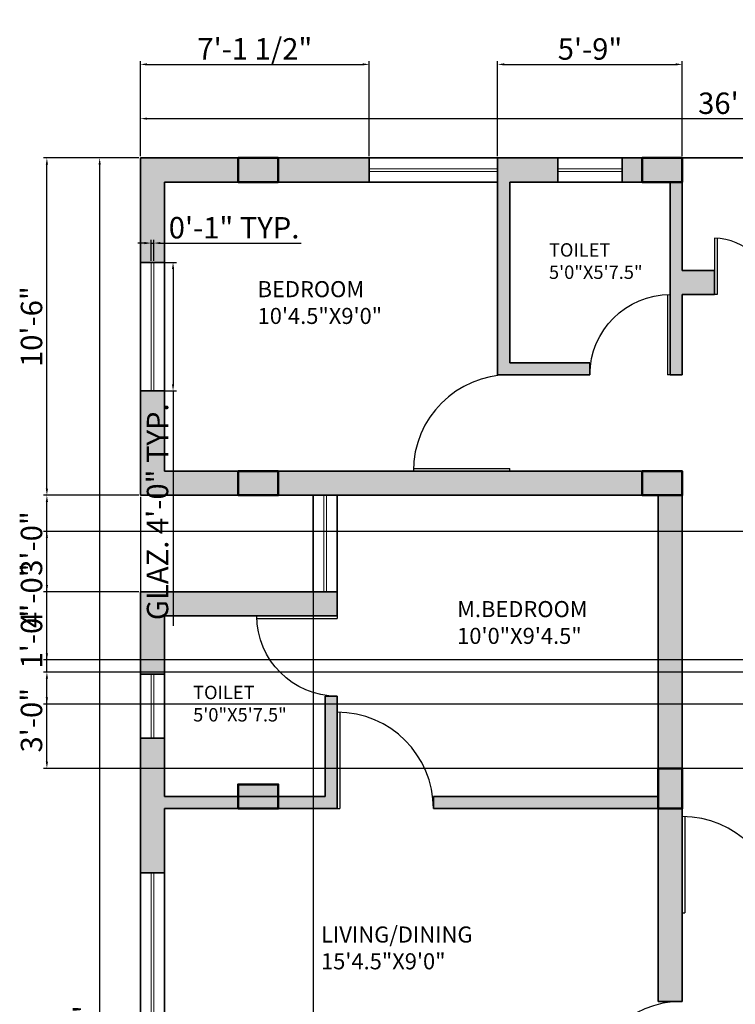
# Model space of a CAD drawing. Units: inches. Extents: x 3010 to 3575, y 2253 to 2995.
# Tile 3 of 4: x 3010 to 3278, y 2627 to 2995. Entities that reach past the tile are written whole.
import ezdxf

# ---------------------------------------------------------------- set-up
doc = ezdxf.new("R2010")
doc.units = ezdxf.units.IN
for name, color, linetype, lineweight in [('A-ANNO-DIMS', 2, 'Continuous', 18), ('A-AREA-IDEN', 7, 'Continuous', 18), ('A-COLS', 7, 'Continuous', 50), ('A-COLS-PATT', 1, 'Continuous', 13), ('A-DOOR', 3, 'Continuous', 25), ('A-GLAZ', 4, 'Continuous', 18), ('A-WALL', 7, 'Continuous', 35)]:
    doc.layers.add(name, color=color, linetype=linetype, lineweight=lineweight)
doc.layers.add('A-WALL-PATT', color=9, linetype='Continuous', lineweight=13, true_color=0xc7c8ca)
doc.styles.get("Standard").update_dxf_attribs({"font": 'arial.ttf'})
doc.dimstyles.new('ISO-25', dxfattribs={"dimtxt": 8, "dimasz": 2.5, "dimexe": 1.25, "dimexo": 0.625, "dimtad": 1, "dimdec": 1, "dimlunit": 3, "dimtxsty": 'Standard', "dimcen": 2.5, "dimadec": 0, "dimazin": 0, "dimtfac": 1, "dimtdec": 1, "dimtmove": 0, "dimatfit": 3, "dimfxl": 1, "dimarcsym": 0})

# ---------------------------------------------------------------- blocks, each defined once
blk = doc.blocks.new('*D1')
at = {"layer": 'A-ANNO-DIMS', "color": 0, "lineweight": -2, "transparency": 16777216}
for p, q in [((3055.45, 2944.01), (3055.45, 2959.31)), ((3057.95, 2958.06), (3484.95, 2958.06)), ((3487.45, 2944.01), (3487.45, 2959.31))]:
    blk.add_line(p, q, dxfattribs=at)
at = {"layer": 'A-ANNO-DIMS', "color": 0, "transparency": 16777216}
for points in [[(3057.95, 2958.48), (3057.95, 2957.65), (3055.45, 2958.06)], [(3484.95, 2958.48), (3484.95, 2957.65), (3487.45, 2958.06)]]:
    blk.add_solid(points, dxfattribs=at)
at = {"layer": 'Defpoints', "color": 0, "transparency": 16777216}
for p in [(3487.45, 2958.06), (3055.45, 2943.38), (3487.45, 2943.38)]:
    blk.add_point(p, dxfattribs=at)
at = {"layer": 'A-ANNO-DIMS', "color": 0, "transparency": 16777216, "insert": (3271.45, 2962.78), "char_height": 8, "attachment_point": 5}
blk.add_mtext("36'", dxfattribs=at)
blk = doc.blocks.new('*D2')
at = {"layer": 'A-ANNO-DIMS', "color": 0, "lineweight": -2, "transparency": 16777216}
for p, q in [((3054.82, 2943.38), (3038.98, 2943.38)), ((3040.23, 2297.88), (3040.23, 2940.88)), ((3054.82, 2295.38), (3038.98, 2295.38))]:
    blk.add_line(p, q, dxfattribs=at)
at = {"layer": 'A-ANNO-DIMS', "color": 0, "transparency": 16777216}
for points in [[(3039.81, 2940.88), (3040.64, 2940.88), (3040.23, 2943.38)], [(3039.81, 2297.88), (3040.64, 2297.88), (3040.23, 2295.38)]]:
    blk.add_solid(points, dxfattribs=at)
at = {"layer": 'Defpoints', "color": 0, "transparency": 16777216}
for p in [(3040.23, 2943.38), (3055.45, 2943.38), (3055.45, 2295.38)]:
    blk.add_point(p, dxfattribs=at)
at = {"layer": 'A-ANNO-DIMS', "color": 0, "transparency": 16777216, "insert": (3035.53, 2619.38), "char_height": 8, "attachment_point": 5, "rotation": 90}
blk.add_mtext("54'", dxfattribs=at)
blk = doc.blocks.new("D1 3'")
for p, q in [((0, 36), (0, 0)), ((1, 36), (1, 0)), ((0, 0), (1, 0))]:
    blk.add_line(p, q)
blk.add_arc((0, 0), 36, 0, 90)
blk = doc.blocks.new("D2 2'6")
for p, q in [((0, 30), (0, 0)), ((1, 30), (1, 0)), ((0, 0), (1, 0))]:
    blk.add_line(p, q)
blk.add_arc((0, 0), 30, 0, 90)
blk = doc.blocks.new('FLOD D')
for p, q in [((3539.49, 2401.61), (3539.49, 2380.61)), ((3540.49, 2401.61), (3540.49, 2380.61)), ((3560.49, 2401.61), (3560.49, 2380.61)), ((3561.49, 2401.61), (3561.49, 2380.61)), ((3601.49, 2401.61), (3601.49, 2380.61)), ((3602.49, 2401.61), (3602.49, 2380.61)), ((3622.49, 2401.61), (3622.49, 2380.61)), ((3623.49, 2401.61), (3623.49, 2380.61)), ((3540.49, 2380.61), (3539.49, 2380.61)), ((3561.49, 2380.61), (3560.49, 2380.61)), ((3602.49, 2380.61), (3601.49, 2380.61)), ((3623.49, 2380.61), (3622.49, 2380.61))]:
    blk.add_line(p, q)
for centre, start, end in [((3539.49, 2380.61), 0, 90), ((3560.49, 2380.61), 0, 90), ((3602.49, 2380.61), 90, 180), ((3623.49, 2380.61), 90, 180)]:
    blk.add_arc(centre, 21, start, end)
blk = doc.blocks.new('GLAZING-24IN')
for p, q in [((24, 1), (0, 1)), ((24, 0), (0, 0))]:
    blk.add_line(p, q)
blk = doc.blocks.new('GLAZING-36IN')
for p, q in [((36, 1), (0, 1)), ((36, 0), (0, 0))]:
    blk.add_line(p, q)
blk = doc.blocks.new('GLAZING-48IN')
for p, q in [((48, 1), (0, 1)), ((48, 0), (0, 0))]:
    blk.add_line(p, q)
blk = doc.blocks.new('GLAZING-60IN')
for p, q in [((0, 0), (0, 60)), ((1, 0), (1, 60))]:
    blk.add_line(p, q)
blk = doc.blocks.new('*D19')
at = {"layer": 'A-ANNO-DIMS', "color": 0, "lineweight": -2, "transparency": 16777216}
for p, q in [((3061.07, 2904.38), (3068.9, 2904.38)), ((3067.65, 2901.88), (3067.65, 2858.88)), ((3061.07, 2856.38), (3068.9, 2856.38)), ((3067.65, 2856.38), (3067.65, 2768.6))]:
    blk.add_line(p, q, dxfattribs=at)
at = {"layer": 'A-ANNO-DIMS', "color": 0, "transparency": 16777216}
for points in [[(3067.23, 2901.88), (3068.06, 2901.88), (3067.65, 2904.38)], [(3067.23, 2858.88), (3068.06, 2858.88), (3067.65, 2856.38)]]:
    blk.add_solid(points, dxfattribs=at)
at = {"layer": 'Defpoints', "color": 0, "transparency": 16777216}
for p in [(3060.45, 2904.38), (3060.45, 2856.38), (3067.65, 2856.38)]:
    blk.add_point(p, dxfattribs=at)
at = {"layer": 'A-ANNO-DIMS', "color": 0, "transparency": 16777216, "insert": (3062.88, 2811.24), "char_height": 8, "attachment_point": 5, "rotation": 90}
blk.add_mtext('GLAZ. 4\'-0" TYP.', dxfattribs=at)
blk = doc.blocks.new('*D20')
at = {"layer": 'A-ANNO-DIMS', "color": 0, "lineweight": -2, "transparency": 16777216}
for p, q in [((3059.45, 2905.01), (3059.45, 2912.83)), ((3060.45, 2905.01), (3060.45, 2912.83)), ((3056.95, 2911.58), (3054.45, 2911.58)), ((3059.45, 2911.58), (3060.45, 2911.58)), ((3062.95, 2911.58), (3115.46, 2911.58))]:
    blk.add_line(p, q, dxfattribs=at)
at = {"layer": 'A-ANNO-DIMS', "color": 0, "transparency": 16777216}
for points in [[(3056.95, 2912), (3056.95, 2911.17), (3059.45, 2911.58)], [(3062.95, 2912), (3062.95, 2911.17), (3060.45, 2911.58)]]:
    blk.add_solid(points, dxfattribs=at)
at = {"layer": 'Defpoints', "color": 0, "transparency": 16777216}
for p in [(3060.45, 2911.58), (3059.45, 2904.38), (3060.45, 2904.38)]:
    blk.add_point(p, dxfattribs=at)
at = {"layer": 'A-ANNO-DIMS', "color": 0, "transparency": 16777216, "insert": (3090.45, 2916.29), "char_height": 8, "attachment_point": 5}
blk.add_mtext('0\'-1" TYP.', dxfattribs=at)
blk = doc.blocks.new('*D40')
at = {"layer": 'A-ANNO-DIMS', "color": 0, "lineweight": -2, "transparency": 16777216}
for p, q in [((3389.32, 2803.88), (3019.25, 2803.88)), ((3020.5, 2758.38), (3020.5, 2801.38)), ((3389.32, 2755.88), (3019.25, 2755.88))]:
    blk.add_line(p, q, dxfattribs=at)
at = {"layer": 'A-ANNO-DIMS', "color": 0, "transparency": 16777216}
for points in [[(3020.08, 2801.38), (3020.91, 2801.38), (3020.5, 2803.88)], [(3020.08, 2758.38), (3020.91, 2758.38), (3020.5, 2755.88)]]:
    blk.add_solid(points, dxfattribs=at)
at = {"layer": 'Defpoints', "color": 0, "transparency": 16777216}
for p in [(3020.5, 2803.88), (3389.95, 2803.88), (3389.95, 2755.88)]:
    blk.add_point(p, dxfattribs=at)
at = {"layer": 'A-ANNO-DIMS', "color": 0, "transparency": 16777216, "insert": (3015.79, 2779.88), "char_height": 8, "attachment_point": 5, "rotation": 90}
blk.add_mtext('4\'-0"', dxfattribs=at)
blk = doc.blocks.new('*D42')
at = {"layer": 'A-ANNO-DIMS', "color": 0, "lineweight": -2, "transparency": 16777216}
for p, q in [((3365.32, 2751.38), (3019.25, 2751.38)), ((3020.5, 2717.88), (3020.5, 2748.88)), ((3365.32, 2715.38), (3019.25, 2715.38))]:
    blk.add_line(p, q, dxfattribs=at)
at = {"layer": 'A-ANNO-DIMS', "color": 0, "transparency": 16777216}
for points in [[(3020.08, 2748.88), (3020.91, 2748.88), (3020.5, 2751.38)], [(3020.08, 2717.88), (3020.91, 2717.88), (3020.5, 2715.38)]]:
    blk.add_solid(points, dxfattribs=at)
at = {"layer": 'Defpoints', "color": 0, "transparency": 16777216}
for p in [(3020.5, 2751.38), (3365.95, 2751.38), (3365.95, 2715.38)]:
    blk.add_point(p, dxfattribs=at)
at = {"layer": 'A-ANNO-DIMS', "color": 0, "transparency": 16777216, "insert": (3015.78, 2733.38), "char_height": 8, "attachment_point": 5, "rotation": 90}
blk.add_mtext('3\'-0"', dxfattribs=at)
blk = doc.blocks.new('*D43')
at = {"layer": 'A-ANNO-DIMS', "color": 0, "lineweight": -2, "transparency": 16777216}
for p, q in [((3020.5, 2751.38), (3020.5, 2775.65)), ((3411.82, 2751.38), (3019.25, 2751.38)), ((3020.5, 2741.88), (3020.5, 2748.88)), ((3416.32, 2739.38), (3019.25, 2739.38))]:
    blk.add_line(p, q, dxfattribs=at)
at = {"layer": 'A-ANNO-DIMS', "color": 0, "transparency": 16777216}
for points in [[(3020.08, 2748.88), (3020.91, 2748.88), (3020.5, 2751.38)], [(3020.08, 2741.88), (3020.91, 2741.88), (3020.5, 2739.38)]]:
    blk.add_solid(points, dxfattribs=at)
at = {"layer": 'Defpoints', "color": 0, "transparency": 16777216}
for p in [(3020.5, 2751.38), (3412.45, 2751.38), (3416.95, 2739.38)]:
    blk.add_point(p, dxfattribs=at)
at = {"layer": 'A-ANNO-DIMS', "color": 0, "transparency": 16777216, "insert": (3015.79, 2764.76), "char_height": 8, "attachment_point": 5, "rotation": 90}
blk.add_mtext('1\'-0"', dxfattribs=at)
blk = doc.blocks.new('*D48')
at = {"layer": 'A-ANNO-DIMS', "color": 0, "lineweight": -2, "transparency": 16777216}
for p, q in [((3188.95, 2944.01), (3188.95, 2979.58)), ((3257.95, 2944.01), (3257.95, 2979.58)), ((3191.45, 2978.33), (3255.45, 2978.33))]:
    blk.add_line(p, q, dxfattribs=at)
at = {"layer": 'A-ANNO-DIMS', "color": 0, "transparency": 16777216}
for points in [[(3191.45, 2978.75), (3191.45, 2977.92), (3188.95, 2978.33)], [(3255.45, 2978.75), (3255.45, 2977.92), (3257.95, 2978.33)]]:
    blk.add_solid(points, dxfattribs=at)
at = {"layer": 'Defpoints', "color": 0, "transparency": 16777216}
for p in [(3257.95, 2978.33), (3188.95, 2943.38), (3257.95, 2943.38)]:
    blk.add_point(p, dxfattribs=at)
at = {"layer": 'A-ANNO-DIMS', "color": 0, "transparency": 16777216, "insert": (3223.45, 2983.04), "char_height": 8, "attachment_point": 5}
blk.add_mtext('5\'-9"', dxfattribs=at)
blk = doc.blocks.new('*D51')
at = {"layer": 'A-ANNO-DIMS', "color": 0, "lineweight": -2, "transparency": 16777216}
for p, q in [((3054.82, 2943.38), (3019.25, 2943.38)), ((3020.5, 2819.88), (3020.5, 2940.88)), ((3054.82, 2817.38), (3019.25, 2817.38))]:
    blk.add_line(p, q, dxfattribs=at)
at = {"layer": 'A-ANNO-DIMS', "color": 0, "transparency": 16777216}
for points in [[(3020.08, 2940.88), (3020.91, 2940.88), (3020.5, 2943.38)], [(3020.08, 2819.88), (3020.91, 2819.88), (3020.5, 2817.38)]]:
    blk.add_solid(points, dxfattribs=at)
at = {"layer": 'Defpoints', "color": 0, "transparency": 16777216}
for p in [(3020.5, 2943.38), (3055.45, 2943.38), (3055.45, 2817.38)]:
    blk.add_point(p, dxfattribs=at)
at = {"layer": 'A-ANNO-DIMS', "color": 0, "transparency": 16777216, "insert": (3015.79, 2880.38), "char_height": 8, "attachment_point": 5, "rotation": 90}
blk.add_mtext('10\'-6"', dxfattribs=at)
blk = doc.blocks.new('*D52')
at = {"layer": 'A-ANNO-DIMS', "color": 0, "lineweight": -2, "transparency": 16777216}
for p, q in [((3054.82, 2817.38), (3019.25, 2817.38)), ((3020.5, 2783.88), (3020.5, 2814.88)), ((3054.82, 2781.38), (3019.25, 2781.38))]:
    blk.add_line(p, q, dxfattribs=at)
at = {"layer": 'A-ANNO-DIMS', "color": 0, "transparency": 16777216}
for points in [[(3020.08, 2814.88), (3020.91, 2814.88), (3020.5, 2817.38)], [(3020.08, 2783.88), (3020.91, 2783.88), (3020.5, 2781.38)]]:
    blk.add_solid(points, dxfattribs=at)
at = {"layer": 'Defpoints', "color": 0, "transparency": 16777216}
for p in [(3020.5, 2817.38), (3055.45, 2817.38), (3055.45, 2781.38)]:
    blk.add_point(p, dxfattribs=at)
at = {"layer": 'A-ANNO-DIMS', "color": 0, "transparency": 16777216, "insert": (3015.78, 2799.38), "char_height": 8, "attachment_point": 5, "rotation": 90}
blk.add_mtext('3\'-0"', dxfattribs=at)
blk = doc.blocks.new('*D53')
at = {"layer": 'A-ANNO-DIMS', "color": 0, "lineweight": -2, "transparency": 16777216}
for p, q in [((3055.45, 2816.76), (3055.45, 2259.18)), ((3119.95, 2816.76), (3119.95, 2259.18)), ((3057.95, 2260.43), (3117.45, 2260.43))]:
    blk.add_line(p, q, dxfattribs=at)
at = {"layer": 'A-ANNO-DIMS', "color": 0, "transparency": 16777216}
for points in [[(3057.95, 2260.85), (3057.95, 2260.02), (3055.45, 2260.43)], [(3117.45, 2260.85), (3117.45, 2260.02), (3119.95, 2260.43)]]:
    blk.add_solid(points, dxfattribs=at)
at = {"layer": 'Defpoints', "color": 0, "transparency": 16777216}
for p in [(3055.45, 2817.38), (3119.95, 2817.38), (3119.95, 2260.43)]:
    blk.add_point(p, dxfattribs=at)
at = {"layer": 'A-ANNO-DIMS', "color": 0, "transparency": 16777216, "insert": (3087.7, 2265.19), "char_height": 8, "attachment_point": 5}
blk.add_mtext('5\'-4 1/2"', dxfattribs=at)
blk = doc.blocks.new('*D55')
at = {"layer": 'A-ANNO-DIMS', "color": 0, "lineweight": -2, "transparency": 16777216}
for p, q in [((3055.45, 2944.01), (3055.45, 2979.58)), ((3140.95, 2944.01), (3140.95, 2979.58)), ((3057.95, 2978.33), (3138.45, 2978.33))]:
    blk.add_line(p, q, dxfattribs=at)
at = {"layer": 'A-ANNO-DIMS', "color": 0, "transparency": 16777216}
for points in [[(3057.95, 2978.75), (3057.95, 2977.92), (3055.45, 2978.33)], [(3138.45, 2978.75), (3138.45, 2977.92), (3140.95, 2978.33)]]:
    blk.add_solid(points, dxfattribs=at)
at = {"layer": 'Defpoints', "color": 0, "transparency": 16777216}
for p in [(3140.95, 2978.33), (3055.45, 2943.38), (3140.95, 2943.38)]:
    blk.add_point(p, dxfattribs=at)
at = {"layer": 'A-ANNO-DIMS', "color": 0, "transparency": 16777216, "insert": (3098.2, 2983.09), "char_height": 8, "attachment_point": 5}
blk.add_mtext('7\'-1 1/2"', dxfattribs=at)

msp = doc.modelspace()

# ---------------------------------------------------------------- hatches: boundary and pattern name
at = {"layer": 'A-COLS-PATT'}
h = msp.add_hatch(color=256, dxfattribs=at)
h.dxf.hatch_style = 1
h.paths.add_polyline_path([(3106.95, 2934.38), (3106.95, 2943.38), (3091.95, 2943.38), (3091.95, 2934.38)])
h = msp.add_hatch(color=256, dxfattribs=at)
h.dxf.hatch_style = 1
h.paths.add_polyline_path([(3257.95, 2934.38), (3257.95, 2943.38), (3242.95, 2943.38), (3242.95, 2934.38)])
h = msp.add_hatch(color=256, dxfattribs=at)
h.dxf.hatch_style = 1
h.paths.add_polyline_path([(3106.95, 2817.38), (3106.95, 2826.38), (3091.95, 2826.38), (3091.95, 2817.38)])
h = msp.add_hatch(color=256, dxfattribs=at)
h.dxf.hatch_style = 1
h.paths.add_polyline_path([(3257.95, 2817.38), (3257.95, 2826.38), (3242.95, 2826.38), (3242.95, 2817.38)])
h = msp.add_hatch(color=256, dxfattribs=at)
h.dxf.hatch_style = 1
h.paths.add_polyline_path([(3248.95, 2700.38), (3257.95, 2700.38), (3257.95, 2715.38), (3248.95, 2715.38)])
h = msp.add_hatch(color=256, dxfattribs=at)
h.dxf.hatch_style = 1
h.paths.add_polyline_path([(3106.95, 2700.38), (3106.95, 2709.38), (3091.95, 2709.38), (3091.95, 2700.38)])
at = {"layer": 'A-WALL-PATT', "transparency": 33554687}
h = msp.add_hatch(color=256, dxfattribs=at)
h.dxf.hatch_style = 1
h.paths.add_polyline_path([(3064.45, 2499.38), (3055.45, 2499.38), (3055.45, 2457.38), (3064.45, 2457.38)])
h.paths.add_polyline_path([(3091.95, 2421.38), (3055.45, 2421.38), (3055.45, 2382.38), (3064.45, 2382.38), (3064.45, 2412.38), (3091.95, 2412.38)])
h.paths.add_polyline_path([(3248.95, 2421.38), (3176.95, 2421.38), (3176.95, 2464.88), (3194.99, 2464.88), (3194.99, 2473.88), (3176.95, 2473.88), (3176.95, 2551.88), (3172.45, 2551.88), (3172.45, 2515.88), (3172.45, 2421.38), (3106.95, 2421.38), (3106.95, 2412.38), (3248.95, 2412.38)])
h.paths.add_polyline_path([(3064.45, 2346.38), (3055.45, 2346.38), (3055.45, 2295.38), (3091.95, 2295.38), (3091.95, 2304.38), (3064.45, 2304.38)])
h.paths.add_polyline_path([(3129.95, 2304.38), (3106.95, 2304.38), (3106.95, 2295.38), (3129.95, 2295.38)])
h.paths.add_polyline_path([(3211.45, 2304.38), (3193.45, 2304.38), (3193.45, 2376.88), (3188.95, 2376.88), (3188.95, 2304.38), (3165.95, 2304.38), (3165.95, 2295.38), (3211.45, 2295.38)])
h.paths.add_polyline_path([(3269.95, 2346.38), (3257.95, 2346.38), (3257.95, 2376.88), (3223.45, 2376.88), (3223.45, 2371.88), (3253.45, 2371.88), (3253.45, 2304.38), (3257.95, 2304.38), (3257.95, 2337.38), (3269.95, 2337.38)])
h.paths.add_polyline_path([(3242.95, 2304.38), (3235.45, 2304.38), (3235.45, 2295.38), (3242.95, 2295.38)])
h.paths.add_polyline_path([(3370.45, 2346.38), (3353.95, 2346.38), (3353.95, 2337.38), (3365.95, 2337.38), (3365.95, 2304.38), (3370.45, 2304.38)])
h.paths.add_polyline_path([(3389.94, 2304.38), (3380.95, 2304.38), (3380.95, 2295.38), (3389.94, 2295.38)], flags=17)
h.paths.add_polyline_path([(3435.95, 2304.38), (3425.94, 2304.38), (3425.94, 2295.38), (3435.95, 2295.38)], flags=17)
h.paths.add_polyline_path([(3487.45, 2401.88), (3478.45, 2401.88), (3478.45, 2389.88), (3394.45, 2389.88), (3394.45, 2442.38), (3380.95, 2442.38), (3380.95, 2437.88), (3389.95, 2437.88), (3389.95, 2389.88), (3365.95, 2389.88), (3365.95, 2385.38), (3412.45, 2385.38), (3412.45, 2373.38), (3416.95, 2373.38), (3416.95, 2385.38), (3478.45, 2385.38), (3478.45, 2304.38), (3450.95, 2304.38), (3450.95, 2295.38), (3487.45, 2295.38)])
h.paths.add_polyline_path([(3487.45, 2478.38), (3478.45, 2478.38), (3478.45, 2442.38), (3450.95, 2442.38), (3450.95, 2437.88), (3478.45, 2437.88), (3478.45, 2425.88), (3487.45, 2425.88)])
h.paths.add_polyline_path([(3435.95, 2442.38), (3424.45, 2442.38), (3424.45, 2437.88), (3435.95, 2437.88)], flags=17)
h.paths.add_polyline_path([(3248.95, 2592.38), (3221.95, 2592.38), (3172.45, 2592.38), (3172.45, 2587.88), (3248.95, 2587.88)])
h.paths.add_polyline_path([(3257.95, 2577.38), (3248.95, 2577.38), (3248.95, 2473.88), (3230.99, 2473.88), (3230.99, 2464.88), (3248.95, 2464.88), (3248.95, 2427.38), (3257.95, 2427.38)])
h.paths.add_polyline_path([(3365.95, 2583.38), (3293.95, 2583.38), (3293.95, 2574.38), (3365.95, 2574.38)])
h.paths.add_polyline_path([(3370.45, 2574.38), (3365.95, 2574.38), (3365.95, 2478.38), (3370.45, 2478.38)])
h.paths.add_polyline_path([(3435.95, 2583.38), (3380.95, 2583.38), (3380.95, 2574.38), (3435.95, 2574.38)])
h.paths.add_polyline_path([(3487.45, 2583.38), (3450.95, 2583.38), (3450.95, 2574.38), (3478.45, 2574.38), (3478.45, 2538.38), (3487.45, 2538.38)])
h.paths.add_polyline_path([(3064.45, 2551.88), (3055.45, 2551.88), (3055.45, 2535.38), (3136.45, 2535.38), (3136.45, 2557.88), (3131.95, 2557.88), (3131.95, 2539.88), (3064.45, 2539.88)])
h.paths.add_polyline_path([(3091.95, 2704.88), (3064.45, 2704.88), (3064.45, 2726.63), (3055.45, 2726.63), (3055.45, 2676.38), (3064.45, 2676.38), (3064.45, 2700.38), (3091.95, 2700.38)])
h.paths.add_polyline_path([(3064.45, 2616.38), (3055.45, 2616.38), (3055.45, 2575.88), (3064.45, 2575.88), (3064.45, 2587.88), (3091.95, 2587.88), (3091.95, 2592.38), (3064.45, 2592.38)])
h.paths.add_polyline_path([(3487.45, 2688.38), (3478.45, 2688.38), (3478.45, 2670.38), (3450.95, 2670.38), (3450.95, 2661.38), (3487.45, 2661.38)])
h.paths.add_polyline_path([(3450.95, 2661.38), (3446.45, 2661.38), (3446.45, 2583.38), (3450.95, 2583.38)])
h.paths.add_polyline_path([(3435.95, 2670.38), (3380.95, 2670.38), (3380.95, 2661.38), (3435.95, 2661.38)])
h.paths.add_polyline_path([(3365.95, 2670.38), (3293.95, 2670.38), (3293.95, 2661.38), (3365.95, 2661.38)])
h.paths.add_polyline_path([(3370.45, 2715.38), (3365.95, 2715.38), (3365.95, 2670.38), (3370.45, 2670.38)])
h.paths.add_polyline_path([(3257.95, 2700.38), (3248.95, 2700.38), (3248.95, 2628.38), (3257.95, 2628.38)])
h.paths.add_polyline_path([(3128.95, 2742.38), (3124.45, 2742.38), (3124.45, 2704.88), (3106.95, 2704.88), (3106.95, 2700.38), (3128.95, 2700.38)])
h.paths.add_polyline_path([(3248.95, 2704.88), (3164.95, 2704.88), (3164.95, 2700.38), (3248.95, 2700.38)])
h.paths.add_polyline_path([(3257.95, 2817.38), (3248.95, 2817.38), (3248.95, 2715.38), (3257.95, 2715.38)])
h.paths.add_polyline_path([(3128.95, 2781.38), (3055.45, 2781.38), (3055.45, 2750.63), (3064.45, 2750.63), (3064.45, 2772.38), (3128.95, 2772.38)])
h.paths.add_polyline_path([(3242.95, 2826.38), (3106.95, 2826.38), (3106.95, 2817.38), (3242.95, 2817.38)])
h.paths.add_polyline_path([(3091.95, 2826.38), (3064.45, 2826.38), (3064.45, 2856.38), (3055.45, 2856.38), (3055.45, 2817.38), (3091.95, 2817.38)])
h.paths.add_polyline_path([(3064.45, 2934.38), (3091.95, 2934.38), (3091.95, 2943.38), (3055.45, 2943.38), (3055.45, 2904.38), (3064.45, 2904.38)])
h.paths.add_polyline_path([(3140.95, 2943.38), (3106.95, 2943.38), (3106.95, 2934.38), (3140.95, 2934.38)])
h.paths.add_polyline_path([(3211.45, 2943.38), (3188.95, 2943.38), (3188.95, 2862.38), (3223.45, 2862.38), (3223.45, 2866.88), (3193.45, 2866.88), (3193.45, 2934.38), (3211.45, 2934.38)])
h.paths.add_polyline_path([(3257.95, 2934.38), (3253.45, 2934.38), (3253.45, 2862.38), (3257.95, 2862.38), (3257.95, 2892.38), (3269.95, 2892.38), (3269.95, 2901.38), (3257.95, 2901.38)])
h.paths.add_polyline_path([(3242.95, 2943.38), (3235.45, 2943.38), (3235.45, 2934.38), (3242.95, 2934.38)])
h.paths.add_polyline_path([(3370.45, 2934.38), (3365.95, 2934.38), (3365.95, 2901.38), (3353.95, 2901.38), (3353.95, 2892.38), (3365.95, 2892.38), (3365.95, 2844.38), (3370.45, 2844.38)])
h.paths.add_polyline_path([(3389.94, 2943.38), (3380.95, 2943.38), (3380.95, 2934.38), (3389.94, 2934.38)])
h.paths.add_polyline_path([(3435.95, 2943.38), (3425.94, 2943.38), (3425.94, 2934.38), (3435.95, 2934.38)])
h.paths.add_polyline_path([(3487.45, 2943.38), (3450.95, 2943.38), (3450.95, 2934.38), (3478.45, 2934.38), (3478.45, 2895.38), (3487.45, 2895.38)])
h.paths.add_polyline_path([(3487.45, 2847.38), (3478.45, 2847.38), (3478.45, 2808.38), (3450.95, 2808.38), (3450.95, 2803.88), (3478.45, 2803.88), (3478.45, 2791.88), (3487.45, 2791.88)])
h.paths.add_polyline_path([(3435.95, 2808.38), (3424.45, 2808.38), (3424.45, 2803.88), (3435.95, 2803.88)])
h.paths.add_polyline_path([(3487.45, 2767.88), (3478.45, 2767.88), (3478.45, 2755.88), (3394.45, 2755.88), (3394.45, 2808.38), (3380.95, 2808.38), (3380.95, 2803.88), (3389.95, 2803.88), (3389.95, 2755.88), (3365.95, 2755.88), (3365.95, 2751.38), (3412.45, 2751.38), (3412.45, 2739.38), (3416.95, 2739.38), (3416.95, 2751.38), (3478.45, 2751.38), (3478.45, 2724.38), (3487.45, 2724.38)])
h.paths.add_polyline_path([(3398.97, 2495.84), (3456.57, 2495.84), (3456.57, 2518.66), (3398.97, 2518.66)], flags=9)

# ---------------------------------------------------------------- linework, layer by layer
at = {"layer": 'A-COLS'}
for points in [[(3091.95, 2934.38), (3091.95, 2943.38), (3106.95, 2943.38), (3106.95, 2934.38)], [(3242.95, 2934.38), (3242.95, 2943.38), (3257.95, 2943.38), (3257.95, 2934.38)], [(3091.95, 2817.38), (3091.95, 2826.38), (3106.95, 2826.38), (3106.95, 2817.38)], [(3242.95, 2817.38), (3242.95, 2826.38), (3257.95, 2826.38), (3257.95, 2817.38)], [(3248.95, 2715.38), (3257.95, 2715.38), (3257.95, 2700.38), (3248.95, 2700.38)], [(3091.95, 2700.38), (3091.95, 2709.38), (3106.95, 2709.38), (3106.95, 2700.38)]]:
    msp.add_lwpolyline(points, close=True, dxfattribs=at)
at = {"layer": 'A-WALL'}
for p, q in [((3055.45, 2943.38), (3487.45, 2943.38)), ((3055.45, 2817.38), (3055.45, 2943.38)), ((3140.95, 2934.38), (3140.95, 2943.38)), ((3188.95, 2862.38), (3188.95, 2943.38)), ((3211.45, 2934.38), (3211.45, 2943.38)), ((3235.45, 2934.38), (3235.45, 2943.38)), ((3257.95, 2901.38), (3257.95, 2943.38)), ((3064.45, 2934.38), (3188.95, 2934.38)), ((3064.45, 2826.38), (3064.45, 2934.38)), ((3193.45, 2934.38), (3253.45, 2934.38)), ((3193.45, 2866.88), (3193.45, 2934.38)), ((3253.45, 2862.38), (3253.45, 2934.38)), ((3064.45, 2904.38), (3055.45, 2904.38)), ((3257.95, 2901.38), (3269.95, 2901.38)), ((3269.95, 2892.38), (3269.95, 2901.38)), ((3257.95, 2862.38), (3257.95, 2892.38)), ((3257.95, 2892.38), (3269.95, 2892.38)), ((3193.45, 2866.88), (3223.45, 2866.88)), ((3223.45, 2862.38), (3223.45, 2866.88)), ((3188.95, 2862.38), (3223.45, 2862.38)), ((3253.45, 2862.38), (3257.95, 2862.38)), ((3064.45, 2856.38), (3055.45, 2856.38)), ((3064.45, 2826.38), (3257.95, 2826.38)), ((3257.95, 2628.38), (3257.95, 2826.38)), ((3055.45, 2817.38), (3248.95, 2817.38)), ((3119.95, 2781.38), (3119.95, 2817.38)), ((3128.95, 2772.38), (3128.95, 2817.38)), ((3248.95, 2704.88), (3248.95, 2817.38)), ((3055.45, 2781.38), (3128.95, 2781.38)), ((3055.45, 2535.38), (3055.45, 2781.38)), ((3064.45, 2704.88), (3064.45, 2772.38)), ((3064.45, 2772.38), (3128.95, 2772.38)), ((3064.45, 2750.63), (3055.45, 2750.63)), ((3124.45, 2704.88), (3124.45, 2742.38)), ((3124.45, 2742.38), (3128.95, 2742.38)), ((3128.95, 2700.38), (3128.95, 2742.38)), ((3064.45, 2726.63), (3055.45, 2726.63)), ((3064.45, 2704.88), (3124.45, 2704.88)), ((3164.95, 2700.38), (3164.95, 2704.88)), ((3164.95, 2704.88), (3248.95, 2704.88)), ((3064.45, 2700.38), (3128.95, 2700.38)), ((3064.45, 2592.38), (3064.45, 2700.38)), ((3164.95, 2700.38), (3248.95, 2700.38)), ((3248.95, 2628.38), (3248.95, 2700.38)), ((3064.45, 2676.38), (3055.45, 2676.38)), ((3248.95, 2628.38), (3257.95, 2628.38))]:
    msp.add_line(p, q, dxfattribs=at)

# ---------------------------------------------------------------- block references
at = {"layer": 'A-DOOR'}
for name, p in [('FLOD D', (-269.55, 511.77)), ("D1 3'", (3128.95, 2700.38)), ("D1 3'", (3257.95, 2661.38))]:
    msp.add_blockref(name, p, dxfattribs=at)
at = {"layer": 'A-DOOR', "xscale": -1}
msp.add_blockref("D2 2'6", (3253.45, 2862.38), dxfattribs=at)
at = {"layer": 'A-DOOR', "rotation": 90}
for p in [(3193.45, 2826.38), (3257.95, 2592.38)]:
    msp.add_blockref("D1 3'", p, dxfattribs=at)
at = {"layer": 'A-DOOR', "xscale": -1, "rotation": 90}
msp.add_blockref("D2 2'6", (3128.95, 2772.38), dxfattribs=at)
at = {"layer": 'A-GLAZ'}
for name, p in [('GLAZING-48IN', (3140.95, 2938.38)), ('GLAZING-24IN', (3211.45, 2938.38)), ('GLAZING-60IN', (3059.45, 2616.38))]:
    msp.add_blockref(name, p, dxfattribs=at)
for name, p, rotation in [('GLAZING-48IN', (3059.45, 2904.38), 269.9999999999989), ('GLAZING-36IN', (3123.95, 2817.38), 269.9999999999986), ('GLAZING-24IN', (3059.45, 2750.63), 270.0000000000001)]:
    msp.add_blockref(name, p, dxfattribs=dict(at, rotation=rotation))

# ---------------------------------------------------------------- texts
at = {"layer": 'A-AREA-IDEN', "attachment_point": 1}
for s, insert, char_height in [('{\\fTimes New Roman|b0|i0|c0|p18;\\P  TOILET\\P  5\'0"X5\'7.5"}', (3205.06, 2919.87), 5), ('{\\fTimes New Roman|b0|i0|c0|p18;\\PBEDROOM \\P10\'4.5"X9\'0"}', (3099.24, 2907.39), 6), ('{\\fTimes New Roman|b0|i0|c0|p18;\\PM.BEDROOM \\P10\'0"X9\'4.5"}', (3173.81, 2787.89), 6), ('{\\fTimes New Roman|b0|i0|c0|p18;\\P  TOILET\\P  5\'0"X5\'7.5"}', (3072.09, 2754.58), 5), ('{\\fTimes New Roman|b0|i0|c0|p18;\\PLIVING/DINING\\P15\'4.5"X9\'0"}', (3122.94, 2666.34), 6)]:
    msp.add_mtext_dynamic_manual_height_columns(s, width=72.5587, gutter_width=12.5, heights=[0], dxfattribs=dict(at, insert=insert, char_height=char_height))

# ---------------------------------------------------------------- dimensions: what is measured, and where the dimension line sits
at = {"layer": 'A-ANNO-DIMS'}
for base, p1, p2, override, picture, middle in [((3140.95, 2978.33), (3055.45, 2943.38), (3140.95, 2943.38), {"dimdec": 1, "dimlfac": 1, "dimrnd": 0, "dimzin": 1, "dimdsep": 46, "dimlunit": 4, "dimfrac": 2}, '*D55', (3098.2, 2983.09)), ((3257.95, 2978.33), (3188.95, 2943.38), (3257.95, 2943.38), {"dimdec": 1, "dimlfac": 1, "dimrnd": 0, "dimzin": 1, "dimdsep": 46, "dimlunit": 4, "dimfrac": 2}, '*D48', (3223.45, 2983.04)), ((3487.45, 2958.06), (3055.45, 2943.38), (3487.45, 2943.38), {"dimclrd": 0, "dimclre": 0, "dimclrt": 0}, '*D1', (3271.45, 2962.78)), ((3119.95, 2260.43), (3055.45, 2817.38), (3119.95, 2817.38), {"dimdec": 1, "dimlfac": 1, "dimrnd": 0, "dimzin": 1, "dimdsep": 46, "dimlunit": 4, "dimfrac": 2}, '*D53', (3087.7, 2265.19))]:
    dim = msp.add_linear_dim(base=base, p1=p1, p2=p2, dimstyle='ISO-25', override=override, dxfattribs=at)
    dim.commit()
    dim.dimension.update_dxf_attribs({"geometry": picture, "text_midpoint": middle})
for base, p1, p2, angle, override, picture, middle in [((3020.5, 2943.38), (3055.45, 2817.38), (3055.45, 2943.38), 90, {"dimdec": 1, "dimlfac": 1, "dimrnd": 0, "dimzin": 1, "dimdsep": 46, "dimlunit": 4, "dimfrac": 2}, '*D51', (3015.79, 2880.38)), ((3040.23, 2943.38), (3055.45, 2295.38), (3055.45, 2943.38), 270, {"dimclrd": 0, "dimclre": 0, "dimclrt": 0}, '*D2', (3035.53, 2619.38)), ((3020.5, 2817.38), (3055.45, 2781.38), (3055.45, 2817.38), 90, {"dimdec": 1, "dimlfac": 1, "dimrnd": 0, "dimzin": 1, "dimdsep": 46, "dimlunit": 4, "dimfrac": 2}, '*D52', (3015.78, 2799.38)), ((3020.5, 2803.88), (3389.95, 2755.88), (3389.95, 2803.88), 90, {"dimdec": 1, "dimlfac": 1, "dimrnd": 0, "dimzin": 1, "dimdsep": 46, "dimlunit": 4, "dimfrac": 2}, '*D40', (3015.79, 2779.88)), ((3020.5, 2751.38), (3416.95, 2739.38), (3412.45, 2751.38), 90, {"dimdec": 1, "dimlfac": 1, "dimrnd": 0, "dimzin": 1, "dimdsep": 46, "dimlunit": 4, "dimfrac": 2}, '*D43', (3015.79, 2764.76)), ((3020.5, 2751.38), (3365.95, 2715.38), (3365.95, 2751.38), 90, {"dimdec": 1, "dimlfac": 1, "dimrnd": 0, "dimzin": 1, "dimdsep": 46, "dimlunit": 4, "dimfrac": 2}, '*D42', (3015.78, 2733.38))]:
    dim = msp.add_linear_dim(base=base, p1=p1, p2=p2, angle=angle, dimstyle='ISO-25', override=override, dxfattribs=at)
    dim.commit()
    dim.dimension.update_dxf_attribs({"geometry": picture, "text_midpoint": middle})
dim = msp.add_linear_dim(base=(3060.45, 2911.58), p1=(3059.45, 2904.38), p2=(3060.45, 2904.38), text='<> TYP.', dimstyle='ISO-25', override={"dimdec": 1, "dimlfac": 1, "dimrnd": 0, "dimzin": 1, "dimdsep": 46, "dimlunit": 4, "dimfrac": 2}, dxfattribs=at)
dim.commit()
dim.dimension.update_dxf_attribs({"geometry": '*D20', "text_midpoint": (3090.45, 2916.29)})
dim = msp.add_linear_dim(base=(3067.65, 2856.38), p1=(3060.45, 2904.38), p2=(3060.45, 2856.38), angle=270, text='GLAZ. <> TYP.', dimstyle='ISO-25', override={"dimdec": 1, "dimlfac": 1, "dimrnd": 0, "dimzin": 1, "dimdsep": 46, "dimlunit": 4, "dimfrac": 2}, dxfattribs=at)
dim.commit()
dim.dimension.update_dxf_attribs({"geometry": '*D19', "text_midpoint": (3062.88, 2811.24)})

doc.saveas('drawing.dxf')
